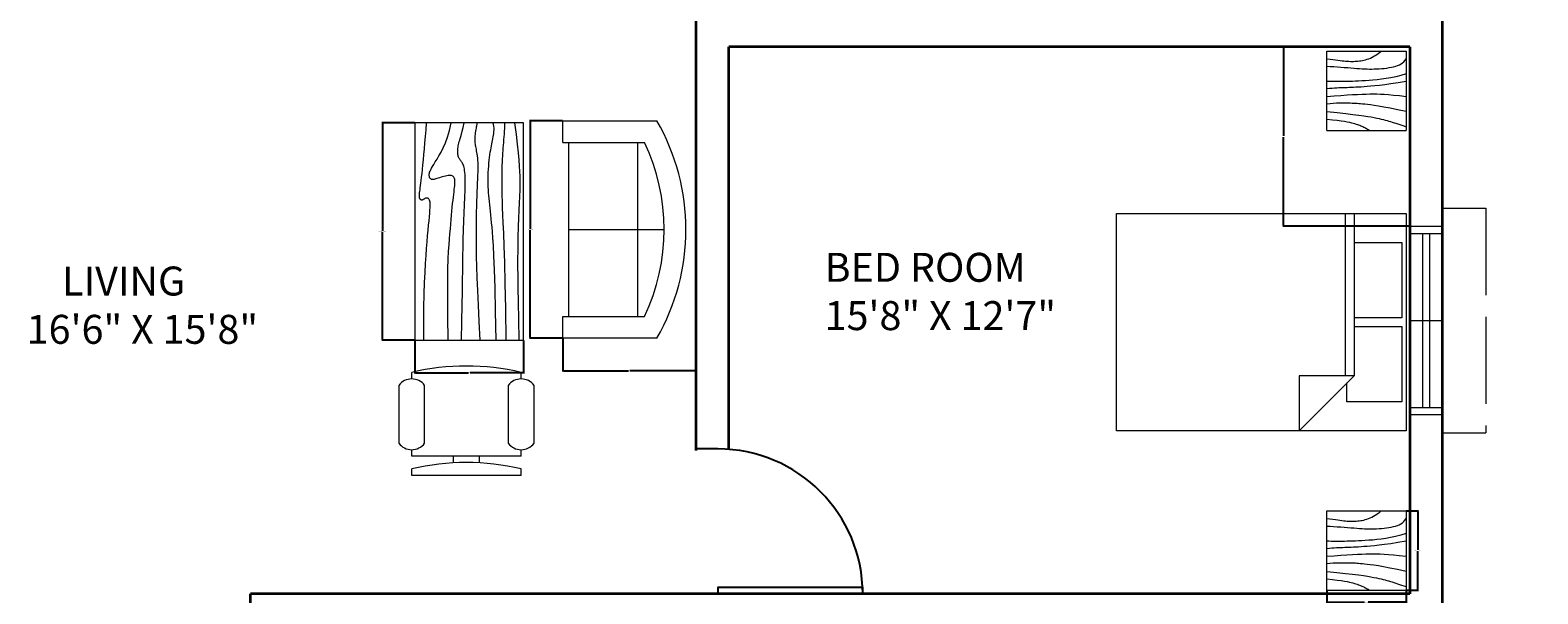
# Model space of a CAD drawing. Units: inches. Extents: x -1138 to 192, y 31 to 760.
# Tile 4 of 6: x -904 to -488, y 323 to 478. Entities that reach past the tile are written whole.
import ezdxf

# ---------------------------------------------------------------- set-up
doc = ezdxf.new("R2010")
doc.units = ezdxf.units.IN
doc.header["$MEASUREMENT"] = 0
doc.linetypes.add('ACAD_ISO02W100', pattern=[15, 12, -3])
for name, color, linetype, lineweight in [('A-ANNO-DIMS', 2, 'Continuous', 18), ('A-AREA-IDEN', 7, 'Continuous', 18), ('A-DOOR', 3, 'Continuous', 25), ('A-FURN', 8, 'Continuous', 18), ('A-GLAZ', 4, 'Continuous', 20), ('A-GLAZ-OVHD', 4, 'ACAD_ISO02W100', 13), ('A-WALL', 7, 'Continuous', 35)]:
    doc.layers.add(name, color=color, linetype=linetype, lineweight=lineweight)
doc.styles.get("Standard").update_dxf_attribs({"font": 'arial.ttf'})
doc.dimstyles.get("Standard").update_dxf_attribs({"dimtxt": 0.18, "dimasz": 0.18, "dimexe": 0.18, "dimexo": 0.0625, "dimgap": 0.09, "dimtad": 0, "dimtih": 1, "dimtoh": 1, "dimdec": 1, "dimzin": 0, "dimdsep": 46, "dimlunit": 4, "dimtxsty": 'Standard', "dimcen": 0.09, "dimadec": 0, "dimazin": 0, "dimtfac": 1, "dimtdec": 1, "dimtofl": 0, "dimtmove": 0, "dimatfit": 3, "dimfxl": 1, "dimtolj": 1, "dimtzin": 0, "dimarcsym": 0})

# ---------------------------------------------------------------- blocks, each defined once
blk = doc.blocks.new('*U4')
for p, q in [((0, 0), (0, -6)), ((-40, 0), (-40, -6))]:
    blk.add_line(p, q)
blk.add_lwpolyline([(0, 0), (0, 40), (-1.75, 40), (-1.75, 0)], close=True)
blk.add_arc((0, 0), 40, 90, 180)
blk = doc.blocks.new('Table - Square Woodgrain 42 x 42 in.')
blk.add_line((0, -42), (42, -42))
for points in [[(0, -4), (1.704, -4.2172), (3.2358, -4.4188), (4.615, -4.604), (5.8615, -4.7721), (6.9951, -4.9224), (8.0357, -5.0541), (9.0031, -5.1667), (9.9171, -5.2594), (10.7951, -5.3316), (11.6445, -5.3836), (12.4702, -5.4157), (13.277, -5.4283), (14.0698, -5.4217), (14.8535, -5.3964), (15.6331, -5.3526), (16.4133, -5.2908), (17.1986, -5.2103), (17.9913, -5.1062), (18.793, -4.9727), (19.6056, -4.8038), (20.4307, -4.5937), (21.2701, -4.3365), (22.1256, -4.0262), (22.9989, -3.6571), (23.888, -3.2272), (24.7756, -2.7516), (25.6408, -2.2491), (26.4624, -1.7387), (27.2195, -1.2395), (27.891, -0.7703), (28.456, -0.3501), (28.8934, 0.002)], [(0, -42), (0, 0), (42, 0), (42, -42)], [(0, -8), (1.8203, -8.1001), (3.6741, -8.2149), (5.5411, -8.3408), (7.4011, -8.4741), (9.2339, -8.6112), (11.0193, -8.7484), (12.7371, -8.8821), (14.3671, -9.0086), (15.8954, -9.1246), (17.3337, -9.2278), (18.6997, -9.3159), (20.0116, -9.387), (21.2871, -9.4389), (22.5442, -9.4696), (23.8008, -9.477), (25.0749, -9.459), (26.3791, -9.4137), (27.7049, -9.3403), (29.0383, -9.2382), (30.3655, -9.1068), (31.6728, -8.9455), (32.9461, -8.7535), (34.1717, -8.5304), (35.3358, -8.2756), (36.4268, -7.9863), (37.443, -7.6521), (38.3849, -7.2603), (39.253, -6.7986), (40.048, -6.2542), (40.7705, -5.6147), (41.421, -4.8674), (42, -4)], [(42, -12), (39.1784, -12.8621), (36.4519, -13.5654), (33.8246, -14.1294), (31.3004, -14.5731), (28.8832, -14.9161), (26.577, -15.1775), (24.3858, -15.3768), (22.3136, -15.5332), (20.3622, -15.6632), (18.5254, -15.7718), (16.7947, -15.8612), (15.1618, -15.9338), (13.6183, -15.9916), (12.1558, -16.0369), (10.7659, -16.0718), (9.4403, -16.0987), (8.1703, -16.1191), (6.9461, -16.1325), (5.7577, -16.1377), (4.595, -16.1335), (3.4479, -16.1188), (2.3064, -16.0924), (1.1604, -16.0532), (0, -16)], [(42, -16), (37.6529, -16.7365), (33.8802, -17.329), (30.6179, -17.7961), (27.8015, -18.1561), (25.3668, -18.4275), (23.2497, -18.6288), (21.3859, -18.7785), (19.7111, -18.8949), (18.1693, -18.9939), (16.7375, -19.0795), (15.401, -19.1534), (14.1449, -19.217), (12.9544, -19.2717), (11.8148, -19.3191), (10.7113, -19.3606), (9.6291, -19.3976), (8.5534, -19.4323), (7.47, -19.4689), (6.3643, -19.5122), (5.222, -19.5672), (4.0288, -19.6386), (2.7703, -19.7313), (1.4321, -19.8501), (0, -20)], [(0, -24), (3.9243, -23.6805), (7.4766, -23.4138), (10.6891, -23.1954), (13.5943, -23.0205), (16.2247, -22.8847), (18.6125, -22.7832), (20.7903, -22.7116), (22.7903, -22.6651), (24.6563, -22.642), (26.4764, -22.6507), (28.35, -22.7024), (30.3766, -22.8084), (32.6555, -22.98), (35.2861, -23.2283), (38.3678, -23.5645), (42, -24)], [(42, -32), (37.392, -31.017), (33.4585, -30.2231), (30.1291, -29.5949), (27.3334, -29.109), (25.0009, -28.742), (23.0612, -28.4707), (21.4439, -28.2716), (20.0786, -28.1215), (18.8998, -28.0002), (17.8609, -27.9014), (16.9206, -27.8219), (16.0371, -27.7588), (15.1691, -27.709), (14.2748, -27.6693), (13.3128, -27.6368), (12.2415, -27.6083), (11.0295, -27.5824), (9.6867, -27.5643), (8.233, -27.5608), (6.6884, -27.5787), (5.0728, -27.6248), (3.4062, -27.7058), (1.7086, -27.8286), (0, -28)], [(0, -32), (5.4026, -32.5358), (9.9494, -33.019), (13.7424, -33.4553), (16.8834, -33.8505), (19.4743, -34.2106), (21.6171, -34.5413), (23.4136, -34.8486), (24.9657, -35.1382), (26.3614, -35.4156), (27.6332, -35.6841), (28.7995, -35.9467), (29.8788, -36.2064), (30.8897, -36.4661), (31.8507, -36.7288), (32.7802, -36.9973), (33.6968, -37.2747), (34.6175, -37.5635), (35.5531, -37.8651), (36.5128, -38.1805), (37.506, -38.5108), (38.5421, -38.8568), (39.6302, -39.2197), (40.7797, -39.6004), (42, -40)], [(0, -36), (3.0098, -36.2857), (5.5354, -36.5643), (7.6368, -36.8359), (9.374, -37.1009), (10.807, -37.3597), (11.9957, -37.6126), (13.0002, -37.8599), (13.8804, -38.102), (14.6874, -38.3393), (15.4365, -38.5729), (16.1338, -38.8041), (16.7858, -39.0341), (17.3987, -39.264), (17.9787, -39.4952), (18.5322, -39.7288), (19.0655, -39.9662), (19.5832, -40.2081), (20.0842, -40.4544), (20.5657, -40.7046), (21.0249, -40.9581), (21.459, -41.2144), (21.8653, -41.4731), (22.2409, -41.7335), (22.5831, -41.9951)]]:
    blk.add_lwpolyline(points)
blk = doc.blocks.new('Bed - Queen')
for p, q in [((0, -80.00003), (0, 0)), ((0, 0), (59.99999, 0)), ((59.99999, 0), (59.99999, -80.00003)), ((7.99999, -1.2), (28.79998, -1.2)), ((7.99999, -14.4), (7.99999, -1.2)), ((28.79998, -1.2), (28.79998, -14.4)), ((31.19999, -1.2), (51.99999, -1.2)), ((31.19999, -14.4), (31.19999, -1.2)), ((51.99999, -1.2), (51.99999, -16.4)), ((0, -14.4), (44.8, -14.4)), ((59.99999, -29.6), (44.8, -14.4)), ((44.8, -14.4), (44.8, -29.6)), ((51.99999, -16.4), (46.79936, -16.4)), ((44.8, -16.8), (0, -16.8)), ((44.8, -29.6), (59.99999, -29.6)), ((59.99999, -80.00003), (0, -80.00003))]:
    blk.add_line(p, q)
blk = doc.blocks.new('Sofa - Roundback Loveseat 5 ft.')
for p, q in [((0, -32.44198), (0, -5.99998)), ((-24, -33.99998), (-24, -11.46958)), ((24.00004, -33.99998), (24.00004, -11.46958)), ((-23.9998, -13.38178), (23.99986, -13.38178)), ((-24, -32.44198), (24.00004, -32.44198))]:
    blk.add_line(p, q)
for points in [[(-24, -33.99998), (-30, -33.99998), (-30, -7.99998)], [(30.00004, -7.99998), (30.00004, -33.99998), (24.00004, -33.99998)]]:
    blk.add_lwpolyline(points)
for centre, radius, start, end in [((0, -60.24998), 60.24998, 60.13715, 119.8628), ((0, -61.38438), 55.38444, 64.32083, 115.6792)]:
    blk.add_arc(centre, radius, start, end)
blk = doc.blocks.new('Chair - Desk')
for p, q in [((-8.5, 0), (-8.5, -1)), ((-8.5, 0), (8.5, 0)), ((8.5, 0), (8.5, -1)), ((-2, -3), (-2, -1.9355)), ((2, -1.9576), (2, -3)), ((-8.5, -3), (-8.5, -4)), ((-8.5, -3), (8.5, -3)), ((8.5, -3), (8.5, -4)), ((-10.5, -5), (-10.5, -14)), ((-6.5, -14), (-6.5, -5)), ((6.5, -5), (6.5, -14)), ((10.5, -14), (10.5, -5)), ((-8.5, -15), (-8.5, -16)), ((8.5, -15), (8.5, -16))]:
    blk.add_line(p, q)
for centre, radius, start, end in [((0, 34.625), 36.625, 256.5803, 283.4197), ((-8.5, -6.5), 2.5, 36.8699, 143.1301), ((8.5, -6.5), 2.5, 36.8699, 143.1301), ((-8.5, -12.5), 2.5, 216.8699, 323.1301), ((8.5, -12.5), 2.5, 216.8699, 323.1301), ((0, 19.625), 36.625, 256.5803, 283.4197)]:
    blk.add_arc(centre, radius, start, end)
blk = doc.blocks.new('Table - Rectangular Woodgrain 60 x 30 in.')
for p, q in [((0, 0), (0, -30)), ((60, 0), (0, 0)), ((60, -30), (60, 0)), ((0, -30), (60, -30))]:
    blk.add_line(p, q)
for points in [[(0, -2.4), (4.8155, -2.418), (9.0302, -2.4688), (12.709, -2.5477), (15.9167, -2.65), (18.7181, -2.7711), (21.1781, -2.9063), (23.3616, -3.0508), (25.3333, -3.2), (27.1477, -3.3495), (28.8172, -3.4958), (30.3437, -3.636), (31.7291, -3.7667), (32.9756, -3.8849), (34.0849, -3.9875), (35.059, -4.0714), (35.9, -4.1334), (36.6114, -4.1711), (37.2041, -4.1854), (37.6906, -4.1779), (38.0833, -4.15), (38.3948, -4.1034), (38.6375, -4.0396), (38.8239, -3.9602), (38.9666, -3.8667), (39.0764, -3.7608), (39.1573, -3.6448), (39.2116, -3.521), (39.2416, -3.3917), (39.2498, -3.2593), (39.2385, -3.1261), (39.21, -2.9944), (39.1666, -2.8667), (39.111, -2.7447), (39.0468, -2.6281), (38.978, -2.5163), (38.9083, -2.4083), (38.8418, -2.3035), (38.7823, -2.201), (38.7337, -2.1001), (38.7, -2), (38.6844, -1.9003), (38.6875, -1.8021), (38.7094, -1.707), (38.75, -1.6167), (38.8094, -1.5326), (38.8875, -1.4563), (38.9844, -1.3893), (39.1, -1.3333), (39.2351, -1.2896), (39.3937, -1.2583), (39.5804, -1.2396), (39.8, -1.2333), (40.057, -1.2396), (40.3562, -1.2583), (40.7023, -1.2896), (41.1, -1.3333), (41.5547, -1.3895), (42.0755, -1.4573), (42.6721, -1.5361), (43.3542, -1.625), (44.1316, -1.7233), (45.014, -1.8302), (46.0114, -1.9449), (47.1333, -2.0667), (48.3862, -2.1947), (49.7625, -2.3281), (51.2513, -2.4663), (52.8416, -2.6083), (54.5226, -2.7535), (56.2833, -2.9011), (58.1127, -3.0501), (60, -3.2)], [(0, -9.2), (6.5759, -9.0858), (11.9385, -9.0365), (16.2527, -9.0418), (19.6833, -9.0917), (22.3952, -9.1759), (24.5531, -9.2844), (26.322, -9.4069), (27.8666, -9.5333), (29.3241, -9.6553), (30.7203, -9.7719), (32.0532, -9.8837), (33.3208, -9.9917), (34.5213, -10.0965), (35.6526, -10.199), (36.7128, -10.2999), (37.7, -10.4), (38.6129, -10.4996), (39.4531, -10.5969), (40.223, -10.6895), (40.925, -10.775), (41.5613, -10.8512), (42.1344, -10.9156), (42.6465, -10.966), (43.1, -11), (43.4976, -11.0158), (43.8437, -11.0136), (44.143, -10.9942), (44.4, -10.9583), (44.6195, -10.9069), (44.8062, -10.8406), (44.9648, -10.7603), (45.1, -10.6667), (45.2155, -10.5598), (45.3114, -10.4365), (45.3871, -10.2929), (45.4416, -10.125), (45.4743, -9.929), (45.4844, -9.7011), (45.4709, -9.4371), (45.4333, -9.1333), (45.3716, -8.7883), (45.2896, -8.4104), (45.1919, -8.0107), (45.0833, -7.6), (44.9685, -7.1893), (44.8521, -6.7896), (44.7388, -6.4117), (44.6333, -6.0667), (44.54, -5.7628), (44.4614, -5.4979), (44.4001, -5.2675), (44.3583, -5.0667), (44.3384, -4.8909), (44.3427, -4.7354), (44.3736, -4.5956), (44.4333, -4.4667), (44.5236, -4.3453), (44.6427, -4.2333), (44.7884, -4.1339), (44.9583, -4.05), (45.1501, -3.9849), (45.3614, -3.9417), (45.59, -3.9234), (45.8333, -3.9333), (46.0915, -3.9749), (46.3734, -4.0531), (46.6906, -4.1736), (47.0542, -4.3417), (47.4756, -4.5629), (47.9661, -4.8427), (48.5372, -5.1866), (49.2, -5.6), (49.9676, -6.0844), (50.8594, -6.625), (51.8965, -7.2031), (53.1, -7.8), (54.491, -8.3969), (56.0906, -8.975), (57.9199, -9.5156), (60, -10)], [(0, -12.8), (5.1847, -12.9322), (9.6213, -13.0323), (13.3963, -13.1059), (16.5958, -13.1583), (19.3063, -13.1952), (21.614, -13.2219), (23.6054, -13.2439), (25.3666, -13.2667), (26.9728, -13.2947), (28.4531, -13.3281), (29.8256, -13.3663), (31.1083, -13.4083), (32.3191, -13.4535), (33.476, -13.501), (34.597, -13.5501), (35.7, -13.6), (36.7984, -13.6497), (37.8875, -13.6979), (38.9578, -13.743), (40, -13.7833), (41.0047, -13.8174), (41.9625, -13.8438), (42.864, -13.8607), (43.7, -13.8667), (44.4631, -13.8604), (45.1552, -13.8417), (45.7801, -13.8104), (46.3416, -13.7667), (46.8439, -13.7104), (47.2906, -13.6417), (47.6858, -13.5604), (48.0333, -13.4667), (48.3375, -13.3608), (48.6042, -13.2448), (48.8396, -13.121), (49.05, -12.9917), (49.2417, -12.8593), (49.4208, -12.7261), (49.5937, -12.5944), (49.7667, -12.4667), (49.9452, -12.3451), (50.1323, -12.2313), (50.3303, -12.1268), (50.5416, -12.0333), (50.7686, -11.9524), (51.0135, -11.8854), (51.2788, -11.8341), (51.5666, -11.8), (51.8785, -11.7843), (52.2116, -11.7865), (52.562, -11.8059), (52.926, -11.8417), (53.2998, -11.8931), (53.6795, -11.9594), (54.0614, -12.0397), (54.4416, -12.1333), (54.8223, -12.2401), (55.2293, -12.3625), (55.6942, -12.5037), (56.2489, -12.6667), (56.9251, -12.8547), (57.7545, -13.0708), (58.7689, -13.3182), (60, -13.6)], [(0, -18), (5.124, -17.7273), (9.6609, -17.5057), (13.6705, -17.3303), (17.2125, -17.1958), (20.3467, -17.0973), (23.1328, -17.0297), (25.6307, -16.9878), (27.9, -16.9667), (29.9928, -16.9617), (31.9302, -16.9703), (33.7254, -16.9907), (35.3917, -17.0208), (36.9423, -17.0588), (38.3906, -17.1026), (39.7499, -17.1503), (41.0333, -17.2), (42.2519, -17.2496), (43.4073, -17.2969), (44.4986, -17.3395), (45.525, -17.375), (46.4858, -17.4012), (47.3802, -17.4156), (48.2074, -17.416), (48.9667, -17.4), (49.6583, -17.3662), (50.2872, -17.3167), (50.8595, -17.2547), (51.3812, -17.1833), (51.8584, -17.1057), (52.2971, -17.025), (52.7034, -16.9443), (53.0833, -16.8667), (53.443, -16.7951), (53.789, -16.7313), (54.128, -16.6768), (54.4666, -16.6334), (54.8115, -16.6024), (55.1693, -16.5854), (55.5465, -16.5841), (55.95, -16.6), (56.3828, -16.6337), (56.8346, -16.6823), (57.2915, -16.7418), (57.7396, -16.8084), (58.165, -16.878), (58.5539, -16.9469), (58.8924, -17.0111), (59.1666, -17.0667), (59.3679, -17.1107), (59.5078, -17.1438), (59.6032, -17.1675), (59.6708, -17.1833), (59.7275, -17.193), (59.7901, -17.1979), (59.8753, -17.1998), (60, -17.2)], [(0, -22.4), (8.0098, -22.2501), (14.4094, -22.1011), (19.4168, -21.9535), (23.25, -21.8083), (26.1269, -21.6663), (28.2656, -21.5281), (29.884, -21.3947), (31.2, -21.2667), (32.3967, -21.1448), (33.5172, -21.0292), (34.5697, -20.9198), (35.5625, -20.8167), (36.5037, -20.7198), (37.4015, -20.6292), (38.2642, -20.5448), (39.1, -20.4667), (39.9164, -20.3951), (40.7187, -20.3313), (41.5117, -20.2768), (42.3, -20.2333), (43.0883, -20.2024), (43.8812, -20.1854), (44.6836, -20.1841), (45.5, -20.2), (46.3328, -20.234), (47.1747, -20.2844), (48.0163, -20.3488), (48.8479, -20.425), (49.66, -20.5106), (50.4429, -20.6031), (51.1872, -20.7004), (51.8833, -20.8), (52.5246, -20.8999), (53.1166, -20.9995), (53.6681, -21.0983), (54.1875, -21.1958), (54.6834, -21.2919), (55.1646, -21.3859), (55.6394, -21.4777), (56.1167, -21.5667), (56.6028, -21.6515), (57.0961, -21.7266), (57.5929, -21.7852), (58.0896, -21.8208), (58.5823, -21.8268), (59.0674, -21.7964), (59.5412, -21.723), (60, -21.6)], [(0, -25.2), (8.6355, -25.0504), (15.7026, -24.9031), (21.4049, -24.7606), (25.9458, -24.625), (29.529, -24.4988), (32.3578, -24.3844), (34.6359, -24.284), (36.5667, -24.2), (38.3213, -24.1341), (39.9417, -24.0854), (41.437, -24.0523), (42.8167, -24.0333), (44.0901, -24.0268), (45.2667, -24.0313), (46.3557, -24.0451), (47.3667, -24.0667), (48.309, -24.0947), (49.1928, -24.1287), (50.0284, -24.168), (50.826, -24.2125), (51.5959, -24.2617), (52.3483, -24.3151), (53.0935, -24.3725), (53.8417, -24.4334), (54.6009, -24.497), (55.3699, -24.561), (56.1454, -24.6226), (56.9239, -24.6792), (57.7021, -24.7279), (58.4764, -24.7662), (59.2435, -24.7911), (60, -24.8)], [(0, -28.8), (5.6867, -28.6681), (10.45, -28.5698), (14.407, -28.5012), (17.675, -28.4584), (20.3711, -28.4374), (22.6125, -28.4344), (24.5164, -28.4455), (26.2, -28.4667), (27.762, -28.4947), (29.2276, -28.5281), (30.6033, -28.5663), (31.8958, -28.6084), (33.1118, -28.6535), (34.2578, -28.7011), (35.3405, -28.7501), (36.3666, -28.8), (37.3443, -28.8497), (38.288, -28.8974), (39.2137, -28.9412), (40.1375, -28.9792), (41.0753, -29.0093), (42.0432, -29.0297), (43.0572, -29.0384), (44.1333, -29.0333), (45.2936, -29.0114), (46.5843, -28.9641), (48.0579, -28.8816), (49.7666, -28.7542), (51.7629, -28.5721), (54.0989, -28.3255), (56.8272, -28.0048), (60, -27.6)]]:
    blk.add_lwpolyline(points)
blk = doc.blocks.new('WINDOW-48IN')
for p, q in [((0, 0), (0, 9)), ((2, 0), (2, 9)), ((26, 0), (26, 9)), ((50, 0), (50, 9)), ((52, 0), (52, 9)), ((2, 5.5), (50, 5.5)), ((2, 3.5), (50, 3.5))]:
    blk.add_line(p, q)
blk = doc.blocks.new('WINDOW-PROJECTION-62IN')
at = {"ltscale": 2}
for p, q in [((0, 0), (0, 12)), ((0, 12), (62, 12)), ((62, 0), (62, 12)), ((5, 0), (0, 0)), ((57, 0), (62, 0))]:
    blk.add_line(p, q, dxfattribs=at)
blk = doc.blocks.new('*D63')
at = {"layer": 'A-ANNO-DIMS', "color": 0, "lineweight": -2, "transparency": 16777216}
for p, q in [((-524.07, 345.71), (-520.66, 345.71)), ((-520.84, 345.53), (-520.84, 334.93)), ((-520.84, 323.97), (-520.84, 334.56)), ((-524.07, 323.79), (-520.66, 323.79))]:
    blk.add_line(p, q, dxfattribs=at)
at = {"layer": 'A-ANNO-DIMS', "color": 0, "transparency": 16777216}
for points in [[(-520.87, 345.53), (-520.81, 345.53), (-520.84, 345.71)], [(-520.87, 323.97), (-520.81, 323.97), (-520.84, 323.79)]]:
    blk.add_solid(points, dxfattribs=at)
at = {"layer": 'Defpoints', "color": 0, "transparency": 16777216}
for p in [(-524.13, 345.71), (-520.84, 345.71), (-524.13, 323.79)]:
    blk.add_point(p, dxfattribs=at)
at = {"layer": 'A-ANNO-DIMS', "color": 0, "transparency": 16777216, "insert": (-520.84, 334.75), "char_height": 0.18, "attachment_point": 5}
blk.add_mtext('\\A1;SIDE TABLE 22 TYP.', dxfattribs=at)
blk = doc.blocks.new('*D64')
at = {"layer": 'A-ANNO-DIMS', "color": 0, "lineweight": -2, "transparency": 16777216}
for p, q in [((-546.05, 323.73), (-546.05, 320.32)), ((-524.13, 323.73), (-524.13, 320.32)), ((-545.87, 320.5), (-535.62, 320.5)), ((-524.31, 320.5), (-534.56, 320.5))]:
    blk.add_line(p, q, dxfattribs=at)
at = {"layer": 'A-ANNO-DIMS', "color": 0, "transparency": 16777216}
for points in [[(-545.87, 320.53), (-545.87, 320.47), (-546.05, 320.5)], [(-524.31, 320.53), (-524.31, 320.47), (-524.13, 320.5)]]:
    blk.add_solid(points, dxfattribs=at)
at = {"layer": 'Defpoints', "color": 0, "transparency": 16777216}
for p in [(-546.05, 323.79), (-524.13, 323.79), (-524.13, 320.5)]:
    blk.add_point(p, dxfattribs=at)
at = {"layer": 'A-ANNO-DIMS', "color": 0, "transparency": 16777216, "insert": (-535.09, 320.5), "char_height": 0.18, "attachment_point": 5}
blk.add_mtext('\\A1;22 TYP.', dxfattribs=at)
blk = doc.blocks.new('*D81')
at = {"layer": 'A-ANNO-DIMS', "color": 0, "lineweight": -2, "transparency": 16777216}
for p, q in [((-757.01, 453.43), (-766.13, 453.43)), ((-765.95, 453.25), (-765.95, 423.61)), ((-765.95, 393.61), (-765.95, 423.24)), ((-757.01, 393.43), (-766.13, 393.43))]:
    blk.add_line(p, q, dxfattribs=at)
at = {"layer": 'A-ANNO-DIMS', "color": 0, "transparency": 16777216}
for points in [[(-765.98, 453.25), (-765.92, 453.25), (-765.95, 453.43)], [(-765.98, 393.61), (-765.92, 393.61), (-765.95, 393.43)]]:
    blk.add_solid(points, dxfattribs=at)
at = {"layer": 'Defpoints', "color": 0, "transparency": 16777216}
for p in [(-756.95, 453.43), (-765.95, 393.43), (-756.95, 393.43)]:
    blk.add_point(p, dxfattribs=at)
at = {"layer": 'A-ANNO-DIMS', "color": 0, "transparency": 16777216, "insert": (-765.95, 423.43), "char_height": 0.18, "attachment_point": 5}
blk.add_mtext('\\A1;LOVESEAT 60', dxfattribs=at)
blk = doc.blocks.new('*D82')
at = {"layer": 'A-ANNO-DIMS', "color": 0, "lineweight": -2, "transparency": 16777216}
for p, q in [((-756.95, 393.36), (-756.95, 384.25)), ((-720.28, 393.36), (-720.28, 384.25)), ((-756.77, 384.43), (-738.84, 384.43)), ((-720.46, 384.43), (-738.4, 384.43))]:
    blk.add_line(p, q, dxfattribs=at)
at = {"layer": 'A-ANNO-DIMS', "color": 0, "transparency": 16777216}
for points in [[(-756.77, 384.46), (-756.77, 384.4), (-756.95, 384.43)], [(-720.46, 384.46), (-720.46, 384.4), (-720.28, 384.43)]]:
    blk.add_solid(points, dxfattribs=at)
at = {"layer": 'Defpoints', "color": 0, "transparency": 16777216}
for p in [(-756.95, 393.43), (-720.28, 393.43), (-720.28, 384.43)]:
    blk.add_point(p, dxfattribs=at)
at = {"layer": 'A-ANNO-DIMS', "color": 0, "transparency": 16777216, "insert": (-738.62, 384.43), "char_height": 0.18, "attachment_point": 5}
blk.add_mtext('\\A1;37', dxfattribs=at)
blk = doc.blocks.new('*D83')
at = {"layer": 'A-ANNO-DIMS', "color": 0, "lineweight": -2, "transparency": 16777216}
for p, q in [((-797.81, 452.86), (-806.93, 452.86)), ((-806.75, 452.68), (-806.75, 423.04)), ((-806.75, 393.04), (-806.75, 422.67)), ((-797.81, 392.86), (-806.93, 392.86))]:
    blk.add_line(p, q, dxfattribs=at)
at = {"layer": 'A-ANNO-DIMS', "color": 0, "transparency": 16777216}
for points in [[(-806.78, 452.68), (-806.72, 452.68), (-806.75, 452.86)], [(-806.78, 393.04), (-806.72, 393.04), (-806.75, 392.86)]]:
    blk.add_solid(points, dxfattribs=at)
at = {"layer": 'Defpoints', "color": 0, "transparency": 16777216}
for p in [(-806.75, 452.86), (-797.75, 452.86), (-797.75, 392.86)]:
    blk.add_point(p, dxfattribs=at)
at = {"layer": 'A-ANNO-DIMS', "color": 0, "transparency": 16777216, "insert": (-806.75, 422.86), "char_height": 0.18, "attachment_point": 5}
blk.add_mtext('\\A1;COFFEE TABLE 60', dxfattribs=at)
blk = doc.blocks.new('*D84')
at = {"layer": 'A-ANNO-DIMS', "color": 0, "lineweight": -2, "transparency": 16777216}
for p, q in [((-797.75, 392.8), (-797.75, 383.68)), ((-767.75, 392.8), (-767.75, 383.68)), ((-797.57, 383.86), (-782.97, 383.86)), ((-767.93, 383.86), (-782.53, 383.86))]:
    blk.add_line(p, q, dxfattribs=at)
at = {"layer": 'A-ANNO-DIMS', "color": 0, "transparency": 16777216}
for points in [[(-797.57, 383.89), (-797.57, 383.83), (-797.75, 383.86)], [(-767.93, 383.89), (-767.93, 383.83), (-767.75, 383.86)]]:
    blk.add_solid(points, dxfattribs=at)
at = {"layer": 'Defpoints', "color": 0, "transparency": 16777216}
for p in [(-797.75, 392.86), (-767.75, 392.86), (-797.75, 383.86)]:
    blk.add_point(p, dxfattribs=at)
at = {"layer": 'A-ANNO-DIMS', "color": 0, "transparency": 16777216, "insert": (-782.75, 383.86), "char_height": 0.18, "attachment_point": 5}
blk.add_mtext('\\A1;30', dxfattribs=at)
blk = doc.blocks.new('*D86')
at = {"layer": 'A-ANNO-DIMS', "color": 0, "lineweight": -2, "transparency": 16777216}
for p, q in [((-514.07, 700.81), (-467.14, 700.81)), ((-467.32, 700.63), (-467.32, 389.49)), ((-467.32, 77.99), (-467.32, 389.13)), ((-514.07, 77.81), (-467.14, 77.81))]:
    blk.add_line(p, q, dxfattribs=at)
at = {"layer": 'A-ANNO-DIMS', "color": 0, "transparency": 16777216}
for points in [[(-467.35, 700.63), (-467.29, 700.63), (-467.32, 700.81)], [(-467.35, 77.99), (-467.29, 77.99), (-467.32, 77.81)]]:
    blk.add_solid(points, dxfattribs=at)
at = {"layer": 'Defpoints', "color": 0, "transparency": 16777216}
for p in [(-514.13, 700.81), (-467.32, 700.81), (-514.13, 77.81)]:
    blk.add_point(p, dxfattribs=at)
at = {"layer": 'A-ANNO-DIMS', "color": 0, "transparency": 16777216, "insert": (-467.32, 389.31), "char_height": 0.18, "attachment_point": 5}
blk.add_mtext('\\A1;623', dxfattribs=at)
blk = doc.blocks.new('*D96')
at = {"layer": 'A-ANNO-DIMS', "color": 0, "lineweight": -2, "transparency": 16777216}
for p, q in [((-523.2, 473.81), (-558.13, 473.81)), ((-557.95, 473.63), (-557.95, 449.24)), ((-557.95, 424.49), (-557.95, 448.88)), ((-523.2, 424.31), (-558.13, 424.31))]:
    blk.add_line(p, q, dxfattribs=at)
at = {"layer": 'A-ANNO-DIMS', "color": 0, "transparency": 16777216}
for points in [[(-557.98, 473.63), (-557.92, 473.63), (-557.95, 473.81)], [(-557.98, 424.49), (-557.92, 424.49), (-557.95, 424.31)]]:
    blk.add_solid(points, dxfattribs=at)
at = {"layer": 'Defpoints', "color": 0, "transparency": 16777216}
for p in [(-557.95, 473.81), (-523.13, 473.81), (-523.13, 424.31)]:
    blk.add_point(p, dxfattribs=at)
at = {"layer": 'A-ANNO-DIMS', "color": 0, "transparency": 16777216, "insert": (-557.95, 449.06), "char_height": 0.18, "attachment_point": 5}
blk.add_mtext('\\A1;49.5', dxfattribs=at)

msp = doc.modelspace()

# ---------------------------------------------------------------- linework, layer by layer
at = {"layer": 'A-WALL'}
for p, q in [((-720.133, 362.36), (-720.133, 482.813)), ((-514.133, 482.813), (-514.133, 322.813)), ((-523.133, 473.813), (-711.133, 473.813)), ((-711.133, 362.7), (-711.133, 473.813)), ((-523.133, 473.813), (-523.133, 322.813)), ((-523.133, 371.813), (-523.133, 322.813)), ((-514.133, 371.813), (-514.133, 77.813)), ((-720.133, 322.813), (-843.133, 322.813)), ((-843.133, 313.813), (-843.133, 322.813)), ((-523.133, 322.813), (-720.133, 322.813))]:
    msp.add_line(p, q, dxfattribs=at)

# ---------------------------------------------------------------- block references
at = {"layer": 'A-DOOR', "rotation": 270}
msp.add_blockref('*U4', (-714.133, 322.813), dxfattribs=at)
at = {"layer": 'A-FURN', "xscale": 0.5217936972647408, "yscale": 0.5217936972647408, "zscale": 0.5217936972647408}
for p in [(-545.995, 472.67), (-546.047, 345.704)]:
    msp.add_blockref('Table - Square Woodgrain 42 x 42 in.', p, dxfattribs=at)
at = {"layer": 'A-FURN'}
for name, p, rotation in [('Table - Rectangular Woodgrain 60 x 30 in.', (-797.752, 392.858), 90), ('Sofa - Roundback Loveseat 5 ft.', (-722.95, 423.427), 270), ('Bed - Queen', (-524.085, 427.852), 270)]:
    msp.add_blockref(name, p, dxfattribs=dict(at, rotation=rotation))
at = {"layer": 'A-FURN', "xscale": 1.776798148379839, "yscale": 1.776798148379839, "zscale": 1.776798148379839, "rotation": 180}
msp.add_blockref('Chair - Desk', (-783.546, 355.513), dxfattribs=at)
at = {"layer": 'A-GLAZ', "rotation": 270.0000000000001}
msp.add_blockref('WINDOW-48IN', (-523.133, 424.313), dxfattribs=at)
at = {"layer": 'A-GLAZ-OVHD', "rotation": 269.9999999999997}
msp.add_blockref('WINDOW-PROJECTION-62IN', (-514.133, 429.313), dxfattribs=at)

# ---------------------------------------------------------------- texts
at = {"layer": 'A-AREA-IDEN', "char_height": 8, "attachment_point": 1}
for s, insert in [('BED ROOM\\P15\'8" X 12\'7"', (-684.66, 416.974)), ('    LIVING\\P16\'6" X 15\'8"', (-904.958, 413.188))]:
    msp.add_mtext_dynamic_manual_height_columns(s, width=126.58932, gutter_width=1, heights=[0], dxfattribs=dict(at, insert=insert))

# ---------------------------------------------------------------- dimensions: what is measured, and where the dimension line sits
at = {"layer": 'A-ANNO-DIMS'}
for base, p1, p2, angle, override, picture, middle in [((-467.318, 700.813), (-514.133, 77.813), (-514.133, 700.813), 90, {"dimdec": 0, "dimlfac": 1, "dimrnd": 0, "dimzin": 0, "dimdsep": 46, "dimlunit": 2}, '*D86', (-467.318, 389.313)), ((-557.948, 473.813), (-523.133, 424.313), (-523.133, 473.813), 90, {"dimdec": 1, "dimlfac": 1, "dimrnd": 0, "dimzin": 0, "dimdsep": 46, "dimlunit": 2}, '*D96', (-557.948, 449.063)), ((-797.752, 383.858), (-767.752, 392.858), (-797.752, 392.858), 180, {"dimdec": 0, "dimlfac": 1, "dimrnd": 0, "dimzin": 0, "dimdsep": 46, "dimlunit": 2}, '*D84', (-782.752, 383.858))]:
    dim = msp.add_linear_dim(base=base, p1=p1, p2=p2, angle=angle, dimstyle='Standard', override=override, dxfattribs=at)
    dim.commit()
    dim.dimension.update_dxf_attribs({"geometry": picture, "text_midpoint": middle})
for base, p1, p2, angle, text, picture, middle in [((-806.752, 452.858), (-797.752, 392.858), (-797.752, 452.858), 90, 'COFFEE TABLE <>', '*D83', (-806.752, 422.858)), ((-765.95, 393.427), (-756.95, 453.427), (-756.95, 393.427), 270, 'LOVESEAT <>', '*D81', (-765.95, 423.427)), ((-520.844, 345.705), (-524.132, 323.789), (-524.132, 345.705), 90, 'SIDE TABLE <> TYP.', '*D63', (-520.844, 334.747))]:
    dim = msp.add_linear_dim(base=base, p1=p1, p2=p2, angle=angle, text=text, dimstyle='Standard', override={"dimdec": 0, "dimlfac": 1, "dimrnd": 0, "dimzin": 0, "dimdsep": 46, "dimlunit": 2}, dxfattribs=at)
    dim.commit()
    dim.dimension.update_dxf_attribs({"geometry": picture, "text_midpoint": middle})
dim = msp.add_linear_dim(base=(-720.283, 384.427), p1=(-756.95, 393.427), p2=(-720.283, 393.427), dimstyle='Standard', override={"dimdec": 0, "dimlfac": 1, "dimrnd": 0, "dimzin": 0, "dimdsep": 46, "dimlunit": 2}, dxfattribs=at)
dim.commit()
dim.dimension.update_dxf_attribs({"geometry": '*D82', "text_midpoint": (-738.616, 384.427)})
dim = msp.add_linear_dim(base=(-524.132, 320.501), p1=(-546.047, 323.789), p2=(-524.132, 323.789), text='<> TYP.', dimstyle='Standard', override={"dimdec": 0, "dimlfac": 1, "dimrnd": 0, "dimzin": 0, "dimdsep": 46, "dimlunit": 2}, dxfattribs=at)
dim.commit()
dim.dimension.update_dxf_attribs({"geometry": '*D64', "text_midpoint": (-535.089, 320.501)})

doc.saveas('drawing.dxf')
